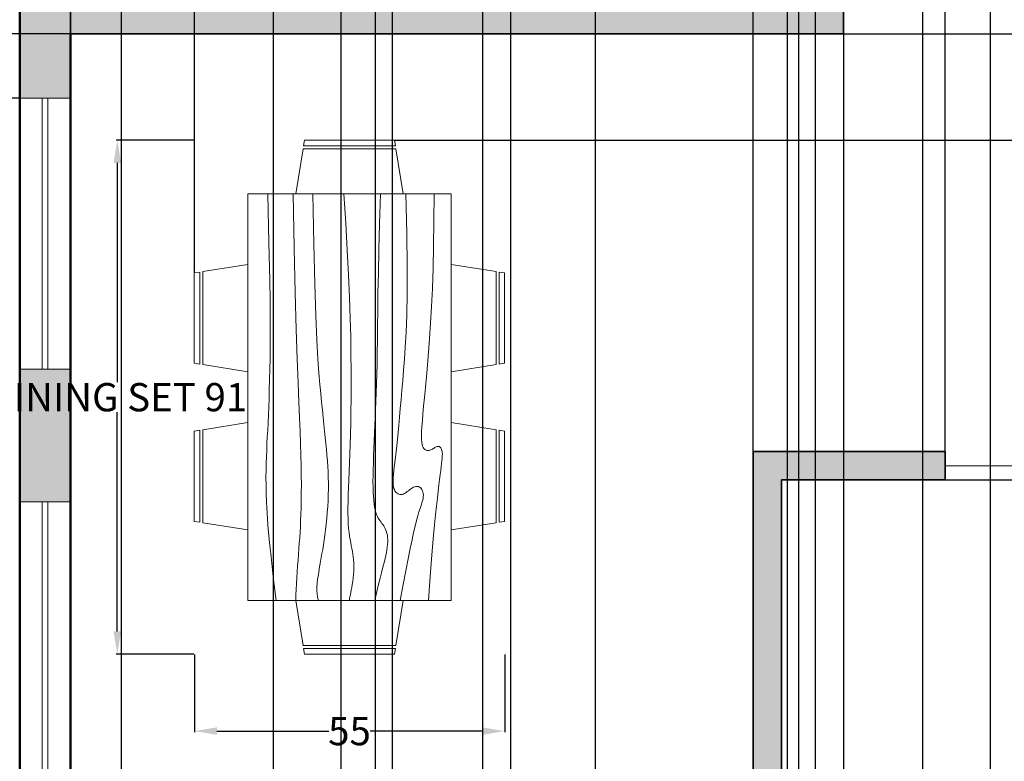
# Model space of a CAD drawing. Units: inches. Extents: x 882 to 1363, y 890 to 1847.
# Tile 4 of 9: x 983 to 1157, y 1220 to 1351. Entities that reach past the tile are written whole.
import ezdxf

# ---------------------------------------------------------------- set-up
doc = ezdxf.new("R2010")
doc.units = ezdxf.units.IN
doc.header["$MEASUREMENT"] = 0
doc.linetypes.add('ACAD_ISO02W100', pattern=[15, 12, -3])
for name, color, linetype, lineweight in [('A-ANNO-DIMS', 2, 'Continuous', 18), ('A-WALL-OVHD', 7, 'ACAD_ISO02W100', 18), ('furniture', 10, 'Continuous', 18), ('inner wall', 50, 'Continuous', 35), ('outer wall', 40, 'Continuous', 50), ('windows', 226, 'Continuous', 18)]:
    doc.layers.add(name, color=color, linetype=linetype, lineweight=lineweight)
doc.layers.add('A-WALL-PATT', color=251, linetype='Continuous', lineweight=13, true_color=0x636466)
doc.styles.get("Standard").update_dxf_attribs({"font": 'arial.ttf'})
doc.dimstyles.get("Standard").update_dxf_attribs({"dimtxt": 5, "dimasz": 4, "dimexe": 0.18, "dimexo": 0.0625, "dimgap": 0.09, "dimtad": 0, "dimtih": 1, "dimtoh": 1, "dimdec": 1, "dimzin": 0, "dimdsep": 46, "dimlunit": 3, "dimtxsty": 'Standard', "dimcen": 0.09, "dimadec": 0, "dimazin": 0, "dimtfac": 1, "dimtdec": 1, "dimtofl": 0, "dimtmove": 0, "dimatfit": 3, "dimfxl": 1, "dimtolj": 1, "dimtzin": 0, "dimarcsym": 0})

# ---------------------------------------------------------------- blocks, each defined once
blk = doc.blocks.new('Dining Set - 36 x 72 in.')
for p, q in [((-22, 27.5), (-22.1562, 26.50042)), ((-5.8416, 26.5), (-22.1534, 26.5)), ((-22, 27.5), (-6, 27.5)), ((-5.8437, 26.49966), (-6, 27.5)), ((6, 27.5), (5.8438, 26.50042)), ((22.1584, 26.5), (5.8466, 26.5)), ((6, 27.5), (22, 27.5)), ((22.1563, 26.49966), (22, 27.5)), ((-22.2343, 26.00059), (-23.4847, 17.99762)), ((-22.2304, 26), (-5.7608, 26)), ((-4.5152, 17.99762), (-5.7655, 25.99926)), ((5.7657, 26.00059), (4.5153, 17.99762)), ((5.7696, 26), (22.2392, 26)), ((23.4848, 17.99762), (22.2345, 25.99926)), ((36, 18), (-36, 18)), ((-36, 18), (-36, -18)), ((36, -18), (36, 18)), ((-44.0006, 8.23428), (-35.9976, 9.48474)), ((44.0006, 8.23428), (35.9976, 9.48474)), ((-45.5, 8), (-44.5004, 8.15617)), ((-45.5, 8), (-45.5, -8)), ((-44.5, -8.15843), (-44.5, 8.15338)), ((-44, 8.23041), (-44, -8.23915)), ((44, 8.23041), (44, -8.23915)), ((44.5, -8.15843), (44.5, 8.15338)), ((45.5, 8), (44.5005, 8.15617)), ((45.5, 8), (45.5, -8)), ((-44.4997, -8.15631), (-45.5, -8)), ((-35.9976, -9.48476), (-43.9993, -8.2345)), ((35.9976, -9.48476), (43.9993, -8.2345)), ((44.4997, -8.15631), (45.5, -8)), ((-36, -18), (36, -18)), ((-22.2343, -26.0006), (-23.4847, -17.99762)), ((-4.5152, -17.99762), (-5.7655, -25.99928)), ((5.7657, -26.0006), (4.5153, -17.99762)), ((23.4848, -17.99762), (22.2345, -25.99928)), ((-22.2304, -26), (-5.7608, -26)), ((5.7696, -26), (22.2392, -26)), ((-22, -27.5), (-22.1562, -26.50044)), ((-5.8416, -26.5), (-22.1534, -26.5)), ((-22, -27.5), (-6, -27.5)), ((-5.8437, -26.49967), (-6, -27.5)), ((6, -27.5), (5.8438, -26.50044)), ((22.1584, -26.5), (5.8466, -26.5)), ((6, -27.5), (22, -27.5)), ((22.1563, -26.49967), (22, -27.5))]:
    blk.add_line(p, q)
for points in [[(-36, 15), (-31.1772, 14.97754), (-26.8079, 14.91406), (-22.8538, 14.81543), (-19.276, 14.6875), (-16.0362, 14.53613), (-13.0957, 14.36718), (-10.4159, 14.18652), (-7.9583, 14), (-5.6904, 13.81315), (-3.6035, 13.63021), (-1.6954, 13.45508), (0.0365, 13.29166), (1.5945, 13.14388), (2.9811, 13.01562), (4.1988, 12.9108), (5.25, 12.83333), (6.1393, 12.78613), (6.8802, 12.76823), (7.4883, 12.77767), (7.9792, 12.8125), (8.3685, 12.87077), (8.6719, 12.95052), (8.9049, 13.0498), (9.0833, 13.16666), (9.2205, 13.29899), (9.3216, 13.44401), (9.3895, 13.59879), (9.4271, 13.76041), (9.4373, 13.92594), (9.4232, 14.09245), (9.3875, 14.257), (9.3333, 14.41666), (9.2638, 14.56917), (9.1836, 14.71484), (9.0975, 14.85465), (9.0104, 14.98958), (8.9272, 15.1206), (8.8529, 15.2487), (8.7922, 15.37483), (8.75, 15.5), (8.7305, 15.62467), (8.7344, 15.74739), (8.7617, 15.86621), (8.8125, 15.97916), (8.8867, 16.08431), (8.9844, 16.17968), (9.1055, 16.26334), (9.25, 16.33333), (9.4189, 16.38802), (9.6172, 16.42708), (9.8506, 16.45052), (10.125, 16.45833), (10.4463, 16.45052), (10.8203, 16.42708), (11.2529, 16.38802), (11.75, 16.33333), (12.3184, 16.26318), (12.9694, 16.17838), (13.7151, 16.07991), (14.5677, 15.96875), (15.5395, 15.84586), (16.6426, 15.71224), (17.8893, 15.56884), (19.2917, 15.41666), (20.859, 15.25667), (22.5879, 15.08984), (24.4721, 14.91715), (26.5052, 14.73958), (28.6809, 14.5581), (30.9929, 14.3737), (33.4347, 14.18733), (36, 14)], [(-36, 10), (-28.9766, 10.14274), (-23.1725, 10.20442), (-18.4241, 10.19775), (-14.5677, 10.13541), (-11.4399, 10.03011), (-8.877, 9.89453), (-6.7154, 9.74137), (-4.7917, 9.58333), (-2.9698, 9.43082), (-1.2246, 9.28515), (0.4415, 9.14534), (2.026, 9.01041), (3.5266, 8.87939), (4.9408, 8.7513), (6.266, 8.62516), (7.5, 8.5), (8.6411, 8.37549), (9.6914, 8.2539), (10.6538, 8.13818), (11.5312, 8.03125), (12.3267, 7.93603), (13.043, 7.85547), (13.6831, 7.79248), (14.25, 7.75), (14.7471, 7.7303), (15.1797, 7.73307), (15.5537, 7.75732), (15.875, 7.80208), (16.1494, 7.86637), (16.3828, 7.94922), (16.5811, 8.04964), (16.75, 8.16666), (16.8944, 8.29915), (17.0143, 8.44531), (17.1089, 8.60319), (17.1771, 8.77083), (17.218, 8.94629), (17.2305, 9.1276), (17.2137, 9.31282), (17.1667, 9.5), (17.0895, 9.6875), (16.987, 9.875), (16.8649, 10.0625), (16.7292, 10.25), (16.5856, 10.4375), (16.4401, 10.625), (16.2985, 10.8125), (16.1667, 11), (16.05, 11.18733), (15.9518, 11.3737), (15.8752, 11.5581), (15.8229, 11.73958), (15.798, 11.91715), (15.8034, 12.08984), (15.842, 12.25667), (15.9167, 12.41666), (16.0295, 12.56836), (16.1784, 12.70833), (16.3605, 12.83268), (16.5729, 12.9375), (16.8127, 13.01888), (17.0768, 13.07291), (17.3625, 13.0957), (17.6667, 13.08333), (17.9894, 13.03312), (18.3418, 12.94726), (18.7382, 12.82918), (19.1927, 12.68229), (19.7195, 12.51001), (20.3327, 12.31575), (21.0465, 12.10294), (21.875, 11.875), (22.8357, 11.63354), (23.959, 11.37304), (25.2786, 11.08618), (26.8282, 10.76562), (28.6414, 10.40405), (30.752, 9.99414), (33.1936, 9.52856), (36, 9)], [(-36, 5.5), (-30.7157, 5.3348), (-26.069, 5.20963), (-21.9946, 5.11767), (-18.4271, 5.05208), (-15.3009, 5.00602), (-12.5508, 4.97265), (-10.1112, 4.94515), (-7.9167, 4.91666), (-5.909, 4.88167), (-4.0586, 4.83984), (-2.3429, 4.79215), (-0.7396, 4.73958), (0.7739, 4.6831), (2.22, 4.6237), (3.6213, 4.56233), (5, 4.5), (6.373, 4.43782), (7.7344, 4.3776), (9.0723, 4.32129), (10.375, 4.27083), (11.6309, 4.22819), (12.8281, 4.19531), (13.9551, 4.17415), (15, 4.16666), (15.954, 4.17448), (16.819, 4.19791), (17.6001, 4.23698), (18.3021, 4.29166), (18.9299, 4.36198), (19.4883, 4.44791), (19.9823, 4.54948), (20.4167, 4.66666), (20.7969, 4.79899), (21.1302, 4.94401), (21.4245, 5.09879), (21.6875, 5.26041), (21.9271, 5.42594), (22.1511, 5.59245), (22.3672, 5.757), (22.5834, 5.91666), (22.8065, 6.06868), (23.0404, 6.21093), (23.2879, 6.34147), (23.5521, 6.45833), (23.8358, 6.55957), (24.142, 6.64323), (24.4735, 6.70735), (24.8334, 6.75), (25.2235, 6.76969), (25.642, 6.76692), (26.0858, 6.74267), (26.5521, 6.69791), (27.0379, 6.63362), (27.5404, 6.55078), (28.0565, 6.45036), (28.5834, 6.33333), (29.1242, 6.19987), (29.7071, 6.04687), (30.3661, 5.87044), (31.1354, 5.66666), (32.0493, 5.43164), (33.142, 5.16146), (34.4475, 4.85221), (36, 4.5)], [(-36, -1), (-30.7915, -0.6591), (-26.0195, -0.38216), (-21.6519, -0.16284), (-17.6563, 0.00521), (-14.0005, 0.12833), (-10.6523, 0.21289), (-7.5796, 0.26522), (-4.75, 0.29166), (-2.134, 0.29793), (0.2878, 0.28711), (2.5317, 0.26163), (4.6146, 0.22396), (6.5529, 0.17651), (8.3633, 0.12174), (10.0623, 0.06209), (11.6667, 0), (13.1899, -0.06201), (14.6341, -0.1211), (15.9982, -0.17432), (17.2813, -0.21875), (18.4823, -0.25147), (19.6003, -0.26953), (20.6343, -0.27002), (21.5834, -0.25), (22.4481, -0.20768), (23.2357, -0.14584), (23.9549, -0.06836), (24.6146, 0.02083), (25.2235, 0.11784), (25.7904, 0.21875), (26.3241, 0.31966), (26.8334, 0.41666), (27.3265, 0.50618), (27.8099, 0.58593), (28.2894, 0.65397), (28.7709, 0.70833), (29.2601, 0.74707), (29.763, 0.76823), (30.2855, 0.76985), (30.8334, 0.75), (31.4088, 0.70784), (31.9994, 0.64713), (32.589, 0.57275), (33.1615, 0.48958), (33.7008, 0.4025), (34.1908, 0.3164), (34.6153, 0.23616), (34.9584, 0.16666), (35.2099, 0.11165), (35.3848, 0.07031), (35.504, 0.04069), (35.5886, 0.02083), (35.6594, 0.00879), (35.7377, 0.0026), (35.8442, 0.00032), (36, 0)], [(-36, -6.5), (-27.1843, -6.31267), (-20.084, -6.1263), (-14.469, -5.9419), (-10.1094, -5.76042), (-6.7752, -5.58285), (-4.2363, -5.41016), (-2.2629, -5.24333), (-0.625, -5.08334), (0.8708, -4.93099), (2.2715, -4.78646), (3.5872, -4.64974), (4.8281, -4.52084), (6.0046, -4.39974), (7.127, -4.28646), (8.2053, -4.18099), (9.25, -4.08334), (10.2705, -3.99382), (11.2734, -3.91407), (12.2647, -3.84603), (13.25, -3.79167), (14.2354, -3.75293), (15.2266, -3.73177), (16.2295, -3.73015), (17.25, -3.75), (18.2912, -3.79248), (19.3451, -3.85547), (20.4009, -3.93604), (21.4479, -4.03125), (22.4754, -4.13819), (23.4727, -4.25391), (24.4289, -4.37549), (25.3334, -4.5), (26.1785, -4.62492), (26.9694, -4.74935), (27.7145, -4.87281), (28.4219, -4.99479), (29.1, -5.11483), (29.7572, -5.23242), (30.4016, -5.34709), (31.0417, -5.45834), (31.6837, -5.56437), (32.3262, -5.65821), (32.9658, -5.73153), (33.599, -5.77604), (34.2224, -5.78345), (34.8327, -5.74545), (35.4264, -5.65373), (36, -5.5)], [(-36, -10), (-26.4022, -9.81299), (-18.4675, -9.62891), (-11.9839, -9.45069), (-6.7396, -9.28125), (-2.5226, -9.12354), (0.8789, -8.98047), (3.6769, -8.85498), (6.0833, -8.75), (8.2767, -8.66765), (10.3021, -8.60677), (12.1712, -8.56543), (13.8958, -8.54167), (15.4876, -8.53353), (16.9583, -8.53907), (18.3197, -8.55632), (19.5834, -8.58334), (20.7616, -8.61841), (21.8685, -8.66081), (22.9188, -8.71004), (23.9271, -8.76563), (24.9081, -8.82707), (25.8763, -8.89388), (26.8465, -8.96558), (27.8334, -9.04167), (28.8474, -9.12118), (29.8828, -9.20117), (30.93, -9.27824), (31.9792, -9.34896), (33.0205, -9.40991), (34.0443, -9.45768), (35.0407, -9.48885), (36, -9.5)], [(-36, -14.5), (-30.0881, -14.33513), (-25.0332, -14.21224), (-20.7312, -14.12647), (-17.0781, -14.07292), (-13.97, -14.04671), (-11.3027, -14.04297), (-8.9724, -14.05681), (-6.875, -14.08334), (-4.9224, -14.11833), (-3.0905, -14.16016), (-1.3709, -14.20785), (0.2448, -14.26042), (1.7647, -14.3169), (3.1973, -14.3763), (4.5507, -14.43767), (5.8333, -14.5), (7.0554, -14.5621), (8.235, -14.62175), (9.3922, -14.67652), (10.5469, -14.72396), (11.7192, -14.76164), (12.929, -14.78711), (14.1965, -14.79794), (15.5417, -14.79167), (16.9933, -14.76424), (18.6152, -14.70508), (20.4804, -14.60197), (22.6615, -14.44271), (25.2312, -14.21509), (28.2624, -13.9069), (31.8277, -13.50594), (36, -13)]]:
    blk.add_lwpolyline(points)
blk = doc.blocks.new('WIN-48IN-9IN')
for p, q in [((4, 0), (4, 48)), ((5, 0), (5, 48))]:
    blk.add_line(p, q)
blk.add_lwpolyline([(0, 48), (9, 48), (9, 0), (0, 0)], close=True)
blk = doc.blocks.new('*D27')
at = {"layer": 'A-ANNO-DIMS', "color": 0, "lineweight": -2, "transparency": 16777216}
for p, q in [((1013.72, 1329.89), (999.96, 1329.89)), ((1000.14, 1325.89), (1000.14, 1287.07)), ((1000.14, 1242.89), (1000.14, 1281.72)), ((1013.72, 1238.89), (999.96, 1238.89))]:
    blk.add_line(p, q, dxfattribs=at)
at = {"layer": 'A-ANNO-DIMS', "color": 0, "transparency": 16777216}
for points in [[(999.47, 1325.89), (1000.8, 1325.89), (1000.14, 1329.89)], [(999.47, 1242.89), (1000.8, 1242.89), (1000.14, 1238.89)]]:
    blk.add_solid(points, dxfattribs=at)
at = {"layer": 'Defpoints', "color": 0, "transparency": 16777216}
for p in [(1013.79, 1329.89), (1000.14, 1238.89), (1013.79, 1238.89)]:
    blk.add_point(p, dxfattribs=at)
at = {"layer": 'A-ANNO-DIMS', "color": 0, "transparency": 16777216, "insert": (1000.14, 1284.39), "char_height": 5, "attachment_point": 5}
blk.add_mtext('\\A1;DINING SET 91', dxfattribs=at)
blk = doc.blocks.new('*D28')
at = {"layer": 'A-ANNO-DIMS', "color": 0, "lineweight": -2, "transparency": 16777216}
for p, q in [((1013.79, 1238.83), (1013.79, 1225.06)), ((1068.79, 1238.83), (1068.79, 1225.06)), ((1017.79, 1225.24), (1037.6, 1225.24)), ((1064.79, 1225.24), (1044.98, 1225.24))]:
    blk.add_line(p, q, dxfattribs=at)
at = {"layer": 'A-ANNO-DIMS', "color": 0, "transparency": 16777216}
for points in [[(1017.79, 1225.91), (1017.79, 1224.58), (1013.79, 1225.24)], [(1064.79, 1225.91), (1064.79, 1224.58), (1068.79, 1225.24)]]:
    blk.add_solid(points, dxfattribs=at)
at = {"layer": 'Defpoints', "color": 0, "transparency": 16777216}
for p in [(1013.79, 1238.89), (1068.79, 1238.89), (1068.79, 1225.24)]:
    blk.add_point(p, dxfattribs=at)
at = {"layer": 'A-ANNO-DIMS', "color": 0, "transparency": 16777216, "insert": (1041.29, 1225.24), "char_height": 5, "attachment_point": 5}
blk.add_mtext('\\A1;55', dxfattribs=at)
blk = doc.blocks.new('*D40')
at = {"layer": 'A-ANNO-DIMS', "color": 0, "lineweight": -2, "transparency": 16777216}
for p, q in [((991.84, 1758.69), (991.84, 893.37)), ((1064.84, 1758.69), (1064.84, 893.37)), ((995.84, 893.55), (1024.69, 893.55)), ((1060.84, 893.55), (1031.99, 893.55))]:
    blk.add_line(p, q, dxfattribs=at)
at = {"layer": 'A-ANNO-DIMS', "color": 0, "transparency": 16777216}
for points in [[(995.84, 894.21), (995.84, 892.88), (991.84, 893.55)], [(1060.84, 894.21), (1060.84, 892.88), (1064.84, 893.55)]]:
    blk.add_solid(points, dxfattribs=at)
at = {"layer": 'Defpoints', "color": 0, "transparency": 16777216}
for p in [(991.84, 1758.75), (1064.84, 1758.75), (1064.84, 893.55)]:
    blk.add_point(p, dxfattribs=at)
at = {"layer": 'A-ANNO-DIMS', "color": 0, "transparency": 16777216, "insert": (1028.34, 893.55), "char_height": 5, "attachment_point": 5}
blk.add_mtext('\\A1;73', dxfattribs=at)
blk = doc.blocks.new('*D41')
at = {"layer": 'A-ANNO-DIMS', "color": 0, "lineweight": -2, "transparency": 16777216}
for p, q in [((1069.84, 1758.69), (1069.84, 893.37)), ((1154.84, 1758.69), (1154.84, 893.37)), ((1073.84, 893.55), (1108.65, 893.55)), ((1150.84, 893.55), (1116.03, 893.55))]:
    blk.add_line(p, q, dxfattribs=at)
at = {"layer": 'A-ANNO-DIMS', "color": 0, "transparency": 16777216}
for points in [[(1073.84, 894.21), (1073.84, 892.88), (1069.84, 893.55)], [(1150.84, 894.21), (1150.84, 892.88), (1154.84, 893.55)]]:
    blk.add_solid(points, dxfattribs=at)
at = {"layer": 'Defpoints', "color": 0, "transparency": 16777216}
for p in [(1069.84, 1758.75), (1154.84, 1758.75), (1154.84, 893.55)]:
    blk.add_point(p, dxfattribs=at)
at = {"layer": 'A-ANNO-DIMS', "color": 0, "transparency": 16777216, "insert": (1112.34, 893.55), "char_height": 5, "attachment_point": 5}
blk.add_mtext('\\A1;85', dxfattribs=at)
blk = doc.blocks.new('*D47')
at = {"layer": 'A-ANNO-DIMS', "color": 0, "lineweight": -2, "transparency": 16777216}
for p, q in [((1123.84, 1567.69), (1123.84, 893.37)), ((1128.84, 1567.69), (1128.84, 893.37)), ((1119.84, 893.55), (1115.84, 893.55)), ((1132.84, 893.55), (1136.84, 893.55))]:
    blk.add_line(p, q, dxfattribs=at)
at = {"layer": 'A-ANNO-DIMS', "color": 0, "transparency": 16777216}
for points in [[(1119.84, 894.21), (1119.84, 892.88), (1123.84, 893.55)], [(1132.84, 894.21), (1132.84, 892.88), (1128.84, 893.55)]]:
    blk.add_solid(points, dxfattribs=at)
at = {"layer": 'Defpoints', "color": 0, "transparency": 16777216}
for p in [(1123.84, 1567.75), (1128.84, 1567.75), (1128.84, 893.55)]:
    blk.add_point(p, dxfattribs=at)
at = {"layer": 'A-ANNO-DIMS', "color": 0, "transparency": 16777216, "insert": (1126.34, 893.55), "char_height": 5, "attachment_point": 5}
blk.add_mtext('\\A1;5', dxfattribs=at)
blk = doc.blocks.new('*D48')
at = {"layer": 'A-ANNO-DIMS', "color": 0, "lineweight": -2, "transparency": 16777216}
for p, q in [((1084.84, 1562.69), (1084.84, 893.37)), ((1120.84, 1562.69), (1120.84, 893.37)), ((1088.84, 893.55), (1099.17, 893.55)), ((1116.84, 893.55), (1106.51, 893.55))]:
    blk.add_line(p, q, dxfattribs=at)
at = {"layer": 'A-ANNO-DIMS', "color": 0, "transparency": 16777216}
for points in [[(1088.84, 894.21), (1088.84, 892.88), (1084.84, 893.55)], [(1116.84, 894.21), (1116.84, 892.88), (1120.84, 893.55)]]:
    blk.add_solid(points, dxfattribs=at)
at = {"layer": 'Defpoints', "color": 0, "transparency": 16777216}
for p in [(1084.84, 1562.75), (1120.84, 1562.75), (1120.84, 893.55)]:
    blk.add_point(p, dxfattribs=at)
at = {"layer": 'A-ANNO-DIMS', "color": 0, "transparency": 16777216, "insert": (1102.84, 893.55), "char_height": 5, "attachment_point": 5}
blk.add_mtext('\\A1;36', dxfattribs=at)
blk = doc.blocks.new('*D51')
at = {"layer": 'A-ANNO-DIMS', "color": 0, "lineweight": -2, "transparency": 16777216}
for p, q in [((982.84, 1767.69), (982.84, 893.37)), ((1000.84, 1767.69), (1000.84, 893.37)), ((986.84, 893.55), (996.84, 893.55)), ((1000.84, 893.55), (1004.84, 893.55))]:
    blk.add_line(p, q, dxfattribs=at)
at = {"layer": 'A-ANNO-DIMS', "color": 0, "transparency": 16777216}
for points in [[(986.84, 894.21), (986.84, 892.88), (982.84, 893.55)], [(996.84, 894.21), (996.84, 892.88), (1000.84, 893.55)]]:
    blk.add_solid(points, dxfattribs=at)
at = {"layer": 'Defpoints', "color": 0, "transparency": 16777216}
for p in [(982.84, 1767.75), (1000.84, 1767.75), (1000.84, 893.55)]:
    blk.add_point(p, dxfattribs=at)
at = {"layer": 'A-ANNO-DIMS', "color": 0, "transparency": 16777216, "insert": (1015.08, 893.55), "char_height": 5, "attachment_point": 5}
blk.add_mtext('\\A1;18.006', dxfattribs=at)
blk = doc.blocks.new('*D52')
at = {"layer": 'A-ANNO-DIMS', "color": 0, "lineweight": -2, "transparency": 16777216}
for p, q in [((1048.84, 1767.69), (1048.84, 893.37)), ((1118.86, 1767.69), (1118.86, 893.37)), ((1052.84, 893.55), (1075.83, 893.55)), ((1114.86, 893.55), (1091.87, 893.55))]:
    blk.add_line(p, q, dxfattribs=at)
at = {"layer": 'A-ANNO-DIMS', "color": 0, "transparency": 16777216}
for points in [[(1052.84, 894.21), (1052.84, 892.88), (1048.84, 893.55)], [(1114.86, 894.21), (1114.86, 892.88), (1118.86, 893.55)]]:
    blk.add_solid(points, dxfattribs=at)
at = {"layer": 'Defpoints', "color": 0, "transparency": 16777216}
for p in [(1048.84, 1767.75), (1118.86, 1767.75), (1118.86, 893.55)]:
    blk.add_point(p, dxfattribs=at)
at = {"layer": 'A-ANNO-DIMS', "color": 0, "transparency": 16777216, "insert": (1083.85, 893.55), "char_height": 5, "attachment_point": 5}
blk.add_mtext('\\A1;70.01', dxfattribs=at)
blk = doc.blocks.new('*D53')
at = {"layer": 'A-ANNO-DIMS', "color": 0, "lineweight": -2, "transparency": 16777216}
for p, q in [((1142.86, 1767.69), (1142.86, 893.37)), ((1171.41, 1767.69), (1171.41, 893.37)), ((1138.86, 893.55), (1134.86, 893.55)), ((1175.41, 893.55), (1179.41, 893.55))]:
    blk.add_line(p, q, dxfattribs=at)
at = {"layer": 'A-ANNO-DIMS', "color": 0, "transparency": 16777216}
for points in [[(1138.86, 894.21), (1138.86, 892.88), (1142.86, 893.55)], [(1175.41, 894.21), (1175.41, 892.88), (1171.41, 893.55)]]:
    blk.add_solid(points, dxfattribs=at)
at = {"layer": 'Defpoints', "color": 0, "transparency": 16777216}
for p in [(1142.86, 1767.75), (1171.41, 1767.75), (1171.41, 893.55)]:
    blk.add_point(p, dxfattribs=at)
at = {"layer": 'A-ANNO-DIMS', "color": 0, "transparency": 16777216, "insert": (1157.14, 893.55), "char_height": 5, "attachment_point": 5}
blk.add_mtext('\\A1;28.554', dxfattribs=at)
blk = doc.blocks.new('*D59')
at = {"layer": 'A-ANNO-DIMS', "color": 0, "lineweight": -2, "transparency": 16777216}
for p, q in [((982.78, 1361.08), (906.46, 1361.08)), ((906.64, 1357.08), (906.64, 1352.75)), ((991.78, 1348.75), (906.46, 1348.75)), ((906.64, 1348.75), (906.64, 1344.75)), ((906.64, 1344.75), (902.64, 1344.75))]:
    blk.add_line(p, q, dxfattribs=at)
at = {"layer": 'A-ANNO-DIMS', "color": 0, "transparency": 16777216}
for points in [[(905.97, 1357.08), (907.3, 1357.08), (906.64, 1361.08)], [(905.97, 1352.75), (907.3, 1352.75), (906.64, 1348.75)]]:
    blk.add_solid(points, dxfattribs=at)
at = {"layer": 'Defpoints', "color": 0, "transparency": 16777216}
for p in [(982.84, 1361.08), (906.64, 1348.75), (991.84, 1348.75)]:
    blk.add_point(p, dxfattribs=at)
at = {"layer": 'A-ANNO-DIMS', "color": 0, "transparency": 16777216, "insert": (892.4, 1344.75), "char_height": 5, "attachment_point": 5}
blk.add_mtext('\\A1;12.328', dxfattribs=at)
blk = doc.blocks.new('*D61')
at = {"layer": 'A-ANNO-DIMS', "color": 0, "lineweight": -2, "transparency": 16777216}
for p, q in [((991.84, 1348.69), (991.84, 893.37)), ((1128.84, 1348.69), (1128.84, 893.37)), ((995.84, 893.55), (1054.96, 893.55)), ((1124.84, 893.55), (1065.72, 893.55))]:
    blk.add_line(p, q, dxfattribs=at)
at = {"layer": 'A-ANNO-DIMS', "color": 0, "transparency": 16777216}
for points in [[(995.84, 894.21), (995.84, 892.88), (991.84, 893.55)], [(1124.84, 894.21), (1124.84, 892.88), (1128.84, 893.55)]]:
    blk.add_solid(points, dxfattribs=at)
at = {"layer": 'Defpoints', "color": 0, "transparency": 16777216}
for p in [(991.84, 1348.75), (1128.84, 1348.75), (1128.84, 893.55)]:
    blk.add_point(p, dxfattribs=at)
at = {"layer": 'A-ANNO-DIMS', "color": 0, "transparency": 16777216, "insert": (1060.34, 893.55), "char_height": 5, "attachment_point": 5}
blk.add_mtext('\\A1;137', dxfattribs=at)
blk = doc.blocks.new('*D62')
at = {"layer": 'A-ANNO-DIMS', "color": 0, "lineweight": -2, "transparency": 16777216}
for p, q in [((991.9, 1348.75), (1353.22, 1348.75)), ((1353.04, 1344.75), (1353.04, 1230.35)), ((1353.04, 1110.75), (1353.04, 1225.15)), ((991.9, 1106.75), (1353.22, 1106.75))]:
    blk.add_line(p, q, dxfattribs=at)
at = {"layer": 'A-ANNO-DIMS', "color": 0, "transparency": 16777216}
for points in [[(1352.38, 1344.75), (1353.71, 1344.75), (1353.04, 1348.75)], [(1352.38, 1110.75), (1353.71, 1110.75), (1353.04, 1106.75)]]:
    blk.add_solid(points, dxfattribs=at)
at = {"layer": 'Defpoints', "color": 0, "transparency": 16777216}
for p in [(991.84, 1348.75), (991.84, 1106.75), (1353.04, 1106.75)]:
    blk.add_point(p, dxfattribs=at)
at = {"layer": 'A-ANNO-DIMS', "color": 0, "transparency": 16777216, "insert": (1353.04, 1227.75), "char_height": 5, "attachment_point": 5}
blk.add_mtext('\\A1;242', dxfattribs=at)
blk = doc.blocks.new('*D64')
at = {"layer": 'A-ANNO-DIMS', "color": 0, "lineweight": -2, "transparency": 16777216}
for p, q in [((1117.84, 1269.69), (1117.84, 893.37)), ((1243.84, 1269.69), (1243.84, 893.37)), ((1121.84, 893.55), (1175.46, 893.55)), ((1239.84, 893.55), (1186.22, 893.55))]:
    blk.add_line(p, q, dxfattribs=at)
at = {"layer": 'A-ANNO-DIMS', "color": 0, "transparency": 16777216}
for points in [[(1121.84, 894.21), (1121.84, 892.88), (1117.84, 893.55)], [(1239.84, 894.21), (1239.84, 892.88), (1243.84, 893.55)]]:
    blk.add_solid(points, dxfattribs=at)
at = {"layer": 'Defpoints', "color": 0, "transparency": 16777216}
for p in [(1117.84, 1269.75), (1243.84, 1269.75), (1243.84, 893.55)]:
    blk.add_point(p, dxfattribs=at)
at = {"layer": 'A-ANNO-DIMS', "color": 0, "transparency": 16777216, "insert": (1180.84, 893.55), "char_height": 5, "attachment_point": 5}
blk.add_mtext('\\A1;126', dxfattribs=at)
blk = doc.blocks.new('*D65')
at = {"layer": 'A-ANNO-DIMS', "color": 0, "lineweight": -2, "transparency": 16777216}
for p, q in [((1117.9, 1269.75), (1353.22, 1269.75)), ((1353.04, 1265.75), (1353.04, 1212.39)), ((1353.04, 1153.75), (1353.04, 1207.11)), ((1117.9, 1149.75), (1353.22, 1149.75))]:
    blk.add_line(p, q, dxfattribs=at)
at = {"layer": 'A-ANNO-DIMS', "color": 0, "transparency": 16777216}
for points in [[(1352.38, 1265.75), (1353.71, 1265.75), (1353.04, 1269.75)], [(1352.38, 1153.75), (1353.71, 1153.75), (1353.04, 1149.75)]]:
    blk.add_solid(points, dxfattribs=at)
at = {"layer": 'Defpoints', "color": 0, "transparency": 16777216}
for p in [(1117.84, 1269.75), (1353.04, 1269.75), (1117.84, 1149.75)]:
    blk.add_point(p, dxfattribs=at)
at = {"layer": 'A-ANNO-DIMS', "color": 0, "transparency": 16777216, "insert": (1353.04, 1209.75), "char_height": 5, "attachment_point": 5}
blk.add_mtext('\\A1;120', dxfattribs=at)
blk = doc.blocks.new('*D68')
at = {"layer": 'A-ANNO-DIMS', "color": 0, "lineweight": -2, "transparency": 16777216}
for p, q in [((1027.84, 1142.81), (1027.84, 1844.13)), ((1031.84, 1843.95), (1066.65, 1843.95)), ((1108.84, 1843.95), (1074.03, 1843.95)), ((1112.84, 1142.81), (1112.84, 1844.13))]:
    blk.add_line(p, q, dxfattribs=at)
at = {"layer": 'A-ANNO-DIMS', "color": 0, "transparency": 16777216}
for points in [[(1031.84, 1844.62), (1031.84, 1843.29), (1027.84, 1843.95)], [(1108.84, 1844.62), (1108.84, 1843.29), (1112.84, 1843.95)]]:
    blk.add_solid(points, dxfattribs=at)
at = {"layer": 'Defpoints', "color": 0, "transparency": 16777216}
for p in [(1112.84, 1843.95), (1027.84, 1142.75), (1112.84, 1142.75)]:
    blk.add_point(p, dxfattribs=at)
at = {"layer": 'A-ANNO-DIMS', "color": 0, "transparency": 16777216, "insert": (1070.34, 1843.95), "char_height": 5, "attachment_point": 5}
blk.add_mtext('\\A1;85', dxfattribs=at)
blk = doc.blocks.new('*D74')
at = {"layer": 'A-ANNO-DIMS', "color": 0, "lineweight": -2, "transparency": 16777216}
for p, q in [((991.84, 1002.81), (991.84, 1844.13)), ((995.84, 1843.95), (1012.06, 1843.95)), ((1035.84, 1843.95), (1019.62, 1843.95)), ((1039.84, 1002.81), (1039.84, 1844.13))]:
    blk.add_line(p, q, dxfattribs=at)
at = {"layer": 'A-ANNO-DIMS', "color": 0, "transparency": 16777216}
for points in [[(995.84, 1844.62), (995.84, 1843.29), (991.84, 1843.95)], [(1035.84, 1844.62), (1035.84, 1843.29), (1039.84, 1843.95)]]:
    blk.add_solid(points, dxfattribs=at)
at = {"layer": 'Defpoints', "color": 0, "transparency": 16777216}
for p in [(1039.84, 1843.95), (991.84, 1002.75), (1039.84, 1002.75)]:
    blk.add_point(p, dxfattribs=at)
at = {"layer": 'A-ANNO-DIMS', "color": 0, "transparency": 16777216, "insert": (1015.84, 1843.95), "char_height": 5, "attachment_point": 5}
blk.add_mtext('\\A1;48', dxfattribs=at)
blk = doc.blocks.new('*D78')
at = {"layer": 'A-ANNO-DIMS', "color": 0, "lineweight": -2, "transparency": 16777216}
for p, q in [((1146.84, 1274.81), (1146.84, 1844.13)), ((1150.84, 1843.95), (1179.69, 1843.95)), ((1215.84, 1843.95), (1186.99, 1843.95)), ((1219.84, 1274.81), (1219.84, 1844.13))]:
    blk.add_line(p, q, dxfattribs=at)
at = {"layer": 'A-ANNO-DIMS', "color": 0, "transparency": 16777216}
for points in [[(1150.84, 1844.62), (1150.84, 1843.29), (1146.84, 1843.95)], [(1215.84, 1844.62), (1215.84, 1843.29), (1219.84, 1843.95)]]:
    blk.add_solid(points, dxfattribs=at)
at = {"layer": 'Defpoints', "color": 0, "transparency": 16777216}
for p in [(1219.84, 1843.95), (1146.84, 1274.75), (1219.84, 1274.75)]:
    blk.add_point(p, dxfattribs=at)
at = {"layer": 'A-ANNO-DIMS', "color": 0, "transparency": 16777216, "insert": (1183.34, 1843.95), "char_height": 5, "attachment_point": 5}
blk.add_mtext('\\A1;73', dxfattribs=at)
blk = doc.blocks.new('*D83')
at = {"layer": 'A-ANNO-DIMS', "color": 0, "lineweight": -2, "transparency": 16777216}
for p, q in [((906.64, 1348.75), (906.64, 1352.75)), ((906.64, 1352.75), (910.64, 1352.75)), ((991.78, 1348.75), (906.46, 1348.75)), ((906.64, 1341.33), (906.64, 1344.75)), ((982.78, 1337.33), (906.46, 1337.33))]:
    blk.add_line(p, q, dxfattribs=at)
at = {"layer": 'A-ANNO-DIMS', "color": 0, "transparency": 16777216}
for points in [[(905.97, 1344.75), (907.3, 1344.75), (906.64, 1348.75)], [(905.97, 1341.33), (907.3, 1341.33), (906.64, 1337.33)]]:
    blk.add_solid(points, dxfattribs=at)
at = {"layer": 'Defpoints', "color": 0, "transparency": 16777216}
for p in [(906.64, 1348.75), (991.84, 1348.75), (982.84, 1337.33)]:
    blk.add_point(p, dxfattribs=at)
at = {"layer": 'A-ANNO-DIMS', "color": 0, "transparency": 16777216, "insert": (920.87, 1352.75), "char_height": 5, "attachment_point": 5}
blk.add_mtext('\\A1;11.416', dxfattribs=at)
blk = doc.blocks.new('*D85')
at = {"layer": 'A-ANNO-DIMS', "color": 0, "lineweight": -2, "transparency": 16777216}
for p, q in [((1045.84, 1562.69), (1045.84, 893.37)), ((1084.84, 1562.69), (1084.84, 893.37)), ((1049.84, 893.55), (1061.66, 893.55)), ((1080.84, 893.55), (1069.01, 893.55))]:
    blk.add_line(p, q, dxfattribs=at)
at = {"layer": 'A-ANNO-DIMS', "color": 0, "transparency": 16777216}
for points in [[(1049.84, 894.21), (1049.84, 892.88), (1045.84, 893.55)], [(1080.84, 894.21), (1080.84, 892.88), (1084.84, 893.55)]]:
    blk.add_solid(points, dxfattribs=at)
at = {"layer": 'Defpoints', "color": 0, "transparency": 16777216}
for p in [(1045.84, 1562.75), (1084.84, 1562.75), (1084.84, 893.55)]:
    blk.add_point(p, dxfattribs=at)
at = {"layer": 'A-ANNO-DIMS', "color": 0, "transparency": 16777216, "insert": (1065.34, 893.55), "char_height": 5, "attachment_point": 5}
blk.add_mtext('\\A1;39', dxfattribs=at)
blk = doc.blocks.new('*D88')
at = {"layer": 'A-ANNO-DIMS', "color": 0, "lineweight": -2, "transparency": 16777216}
for p, q in [((1128.84, 1567.69), (1128.84, 893.37)), ((1211.84, 1562.69), (1211.84, 893.37)), ((1132.84, 893.55), (1166.66, 893.55)), ((1207.84, 893.55), (1174.01, 893.55))]:
    blk.add_line(p, q, dxfattribs=at)
at = {"layer": 'A-ANNO-DIMS', "color": 0, "transparency": 16777216}
for points in [[(1132.84, 894.21), (1132.84, 892.88), (1128.84, 893.55)], [(1207.84, 894.21), (1207.84, 892.88), (1211.84, 893.55)]]:
    blk.add_solid(points, dxfattribs=at)
at = {"layer": 'Defpoints', "color": 0, "transparency": 16777216}
for p in [(1128.84, 1567.75), (1211.84, 1562.75), (1211.84, 893.55)]:
    blk.add_point(p, dxfattribs=at)
at = {"layer": 'A-ANNO-DIMS', "color": 0, "transparency": 16777216, "insert": (1170.34, 893.55), "char_height": 5, "attachment_point": 5}
blk.add_mtext('\\A1;83', dxfattribs=at)
blk = doc.blocks.new('*D89')
at = {"layer": 'A-ANNO-DIMS', "color": 0, "lineweight": -2, "transparency": 16777216}
for p, q in [((991.84, 1473.69), (991.84, 893.37)), ((1084.84, 1473.69), (1084.84, 893.37)), ((995.84, 893.55), (1034.67, 893.55)), ((1080.84, 893.55), (1042.01, 893.55))]:
    blk.add_line(p, q, dxfattribs=at)
at = {"layer": 'A-ANNO-DIMS', "color": 0, "transparency": 16777216}
for points in [[(995.84, 894.21), (995.84, 892.88), (991.84, 893.55)], [(1080.84, 894.21), (1080.84, 892.88), (1084.84, 893.55)]]:
    blk.add_solid(points, dxfattribs=at)
at = {"layer": 'Defpoints', "color": 0, "transparency": 16777216}
for p in [(991.84, 1473.75), (1084.84, 1473.75), (1084.84, 893.55)]:
    blk.add_point(p, dxfattribs=at)
at = {"layer": 'A-ANNO-DIMS', "color": 0, "transparency": 16777216, "insert": (1038.34, 893.55), "char_height": 5, "attachment_point": 5}
blk.add_mtext('\\A1;93', dxfattribs=at)
blk = doc.blocks.new('*D93')
at = {"layer": 'A-ANNO-DIMS', "color": 0, "lineweight": -2, "transparency": 16777216}
for p, q in [((987.84, 1843.95), (983.84, 1843.95)), ((991.84, 1337.4), (991.84, 1844.13)), ((1013.79, 1306.45), (1013.79, 1844.13)), ((1017.79, 1843.95), (1021.79, 1843.95))]:
    blk.add_line(p, q, dxfattribs=at)
at = {"layer": 'A-ANNO-DIMS', "color": 0, "transparency": 16777216}
for points in [[(987.84, 1844.62), (987.84, 1843.29), (991.84, 1843.95)], [(1017.79, 1844.62), (1017.79, 1843.29), (1013.79, 1843.95)]]:
    blk.add_solid(points, dxfattribs=at)
at = {"layer": 'Defpoints', "color": 0, "transparency": 16777216}
for p in [(1013.79, 1843.95), (991.84, 1337.33), (1013.79, 1306.39)]:
    blk.add_point(p, dxfattribs=at)
at = {"layer": 'A-ANNO-DIMS', "color": 0, "transparency": 16777216, "insert": (1002.81, 1843.95), "char_height": 5, "attachment_point": 5}
blk.add_mtext('\\A1;21.95', dxfattribs=at)
blk = doc.blocks.new('*D94')
at = {"layer": 'A-ANNO-DIMS', "color": 0, "lineweight": -2, "transparency": 16777216}
for p, q in [((1128.9, 1348.75), (1353.22, 1348.75)), ((1353.04, 1344.75), (1353.04, 1341.96)), ((1353.04, 1333.89), (1353.04, 1336.68)), ((1049.35, 1329.89), (1353.22, 1329.89))]:
    blk.add_line(p, q, dxfattribs=at)
at = {"layer": 'A-ANNO-DIMS', "color": 0, "transparency": 16777216}
for points in [[(1352.38, 1344.75), (1353.71, 1344.75), (1353.04, 1348.75)], [(1352.38, 1333.89), (1353.71, 1333.89), (1353.04, 1329.89)]]:
    blk.add_solid(points, dxfattribs=at)
at = {"layer": 'Defpoints', "color": 0, "transparency": 16777216}
for p in [(1128.84, 1348.75), (1353.04, 1348.75), (1049.29, 1329.89)]:
    blk.add_point(p, dxfattribs=at)
at = {"layer": 'A-ANNO-DIMS', "color": 0, "transparency": 16777216, "insert": (1353.04, 1339.32), "char_height": 5, "attachment_point": 5}
blk.add_mtext('\\A1;18.858', dxfattribs=at)

msp = doc.modelspace()

# ---------------------------------------------------------------- hatches: boundary and pattern name
at = {"layer": 'A-WALL-PATT'}
h = msp.add_hatch(color=256, dxfattribs=at)
h.dxf.hatch_style = 1
h.paths.add_polyline_path([(1050.8388, 1481.7495), (1050.8388, 1478.7495), (1084.8388, 1478.7495), (1084.8388, 1473.7495), (991.8388, 1473.7495), (991.8388, 1361.0778), (982.8388, 1361.0778), (982.8388, 1556.1531), (991.8388, 1556.1531), (991.8388, 1478.7495), (1045.8388, 1478.7495), (1045.8388, 1481.7479), (1045.4161, 1481.7477), (1030.9055, 1506.8563), (1032.004, 1507.4911), (1046.5146, 1482.3825), (1045.4161, 1481.7477), (1045.8388, 1481.7479), (1045.8388, 1481.7495)])
h.paths.add_polyline_path([(1128.8388, 1478.7495), (1120.8388, 1478.7495), (1120.8388, 1473.7495), (1123.8388, 1473.7495), (1123.8388, 1353.7495), (991.8388, 1353.7495), (991.8388, 1361.0778), (982.8388, 1361.0778), (982.8388, 1337.3333), (991.8388, 1337.3333), (991.8388, 1348.7495), (1128.8388, 1348.7495)])
h.paths.add_polyline_path([(1118.8585, 1767.7495), (1048.8447, 1767.7495), (1048.8447, 1758.7495), (1064.8388, 1758.7495), (1069.8388, 1758.7495), (1118.8585, 1758.7495)])
h.paths.add_polyline_path([(1171.4129, 1767.7495), (1142.8585, 1767.7495), (1142.8585, 1758.7495), (1154.8388, 1758.7495), (1154.8388, 1710.7495), (1069.8388, 1710.7495), (1069.8388, 1713.7495), (1064.8388, 1713.7495), (1064.8388, 1705.7495), (1123.8388, 1705.7495), (1123.8388, 1567.7495), (1120.8388, 1567.7495), (1120.8388, 1562.7495), (1123.8388, 1562.7495), (1211.8388, 1562.7495), (1211.8388, 1567.7495), (1128.8388, 1567.7495), (1128.8388, 1705.7495), (1211.8388, 1705.7495), (1211.8388, 1710.7495), (1159.8388, 1710.7495), (1159.8388, 1758.7495), (1171.4129, 1758.7495)])
h.paths.add_polyline_path([(1252.8388, 1767.7495), (1195.4129, 1767.7495), (1195.4129, 1758.7495), (1243.8388, 1758.7495), (1243.8388, 1710.7495), (1240.8388, 1710.7495), (1240.8388, 1706.4648), (1240.8388, 1705.7495), (1243.8388, 1705.7495), (1243.8388, 1673.1735), (1252.8388, 1673.1735)])
h.paths.add_polyline_path([(1252.8388, 1625.1735), (1243.8388, 1625.1735), (1243.8388, 1567.7495), (1240.8388, 1567.7495), (1240.8388, 1562.7495), (1243.8388, 1562.7495), (1243.8388, 1546.029), (1252.8388, 1546.029)])
h.paths.add_polyline_path([(1252.8388, 1498.029), (1243.8388, 1498.029), (1243.8388, 1391.1399), (1252.8388, 1391.1399)])
h.paths.add_polyline_path([(1252.8388, 1179.8561), (1243.8388, 1179.8561), (1243.8388, 1149.7495), (1219.8388, 1149.7495), (1219.8388, 1145.3111), (1219.8388, 1144.7495), (1252.8388, 1144.7495)])
h.paths.add_polyline_path([(1252.8388, 1277.7495), (1243.8388, 1277.7495), (1243.8388, 1274.7495), (1219.8388, 1274.7495), (1219.8388, 1269.7495), (1243.8388, 1269.7495), (1243.8388, 1227.8561), (1252.8388, 1227.8561)])
h.paths.add_polyline_path([(1252.8388, 1343.1399), (1243.8388, 1343.1399), (1243.8388, 1313.7495), (1248.3388, 1313.7495), (1252.8388, 1313.7495)])
h.paths.add_polyline_path([(1146.8388, 1274.7495), (1112.8388, 1274.7495), (1112.8388, 1106.7495), (1106.7761, 1106.7495), (1106.7761, 1101.7495), (1117.8388, 1101.7495), (1117.8388, 1144.7495), (1159.8388, 1144.7495), (1159.8388, 1149.7495), (1117.8388, 1149.7495), (1117.8388, 1269.7495), (1146.8388, 1269.7495)])
h = msp.add_hatch(color=256, dxfattribs=at)
h.dxf.hatch_style = 1
h.paths.add_polyline_path([(1000.8447, 1767.7495), (993.3979, 1767.7495), (991.8388, 1758.7495), (1000.8447, 1758.7495)])
h.paths.add_polyline_path([(991.8388, 1654.8981), (982.8388, 1654.3544), (982.8388, 1595.0521), (991.8388, 1594.8981)])
h.paths.add_polyline_path([(991.8388, 1594.8981), (982.8388, 1595.0521), (982.8388, 1559.7196), (991.8388, 1562.7495), (991.8388, 1567.7495)])
h.paths.add_polyline_path([(991.8388, 1562.7495), (982.8388, 1559.7196), (982.8388, 1556.1531), (991.8388, 1556.1531)])
h.paths.add_polyline_path([(991.8388, 1289.3333), (982.8388, 1289.3333), (982.8388, 1265.8272), (991.8388, 1265.8272)])
h.paths.add_polyline_path([(1058.7761, 1106.7495), (991.8388, 1106.7495), (982.8388, 1107.8066), (982.8388, 1101.3439), (991.8388, 1101.7495), (1058.7761, 1101.7495)])

# ---------------------------------------------------------------- linework, layer by layer
at = {"layer": 'A-WALL-OVHD'}
msp.add_line((1146.8388, 1272.2495), (1219.8388, 1272.2495), dxfattribs=at)
at = {"layer": 'inner wall'}
for p, q in [((1128.8388, 1348.7495), (1128.8388, 1478.7495)), ((991.8388, 1348.7495), (1128.8388, 1348.7495)), ((1112.8388, 1274.7495), (1146.8388, 1274.7495)), ((1112.8388, 1274.7495), (1112.8388, 1106.7495)), ((1146.8388, 1274.7495), (1146.8388, 1269.7495)), ((1117.8388, 1269.7495), (1146.8388, 1269.7495)), ((1117.8388, 1269.7495), (1117.8388, 1149.7495))]:
    msp.add_line(p, q, dxfattribs=at)
at = {"layer": 'outer wall'}
for p, q in [((982.8388, 993.7495), (982.8388, 1767.7495)), ((991.8388, 1106.7495), (991.8388, 1348.7495))]:
    msp.add_line(p, q, dxfattribs=at)

# ---------------------------------------------------------------- block references
at = {"layer": 'furniture', "rotation": 270}
msp.add_blockref('Dining Set - 36 x 72 in.', (1041.2874, 1284.3919), dxfattribs=at)
at = {"layer": 'windows'}
for p in [(982.839, 1289.3335), (982.839, 1217.8274)]:
    msp.add_blockref('WIN-48IN-9IN', p, dxfattribs=at)

# ---------------------------------------------------------------- dimensions: what is measured, and where the dimension line sits
at = {"layer": 'A-ANNO-DIMS'}
for base, p1, p2, override, picture, middle in [((1013.7874, 1843.953), (991.8388, 1337.3333), (1013.7874, 1306.3919), {"dimdec": 2, "dimlfac": 1, "dimrnd": 0, "dimzin": 0, "dimdsep": 46, "dimlunit": 2}, '*D93', (1002.8131, 1843.953)), ((1039.8388, 1843.953), (991.8388, 1002.7495), (1039.8388, 1002.7495), {"dimdec": 0, "dimlfac": 1, "dimrnd": 0, "dimzin": 0, "dimdsep": 46, "dimlunit": 2}, '*D74', (1015.8388, 1843.953)), ((1112.8388, 1843.953), (1027.8388, 1142.7495), (1112.8388, 1142.7495), {"dimdec": 0, "dimlfac": 1, "dimrnd": 0, "dimzin": 0, "dimdsep": 46, "dimlunit": 2}, '*D68', (1070.3388, 1843.953)), ((1219.8388, 1843.953), (1146.8388, 1274.7495), (1219.8388, 1274.7495), {"dimdec": 0, "dimlfac": 1, "dimrnd": 0, "dimzin": 0, "dimdsep": 46, "dimlunit": 2}, '*D78', (1183.3388, 1843.953)), ((1000.8447, 893.546), (982.8388, 1767.7495), (1000.8447, 1767.7495), {"dimdec": 3, "dimlfac": 1, "dimrnd": 0, "dimzin": 0, "dimdsep": 46, "dimlunit": 2}, '*D51', (1015.0762, 893.546)), ((1118.8585, 893.546), (1048.8447, 1767.7495), (1118.8585, 1767.7495), {"dimdec": 2, "dimlfac": 1, "dimrnd": 0, "dimzin": 0, "dimdsep": 46, "dimlunit": 2}, '*D52', (1083.8516, 893.546)), ((1171.4129, 893.546), (1142.8585, 1767.7495), (1171.4129, 1767.7495), {"dimdec": 3, "dimlfac": 1, "dimrnd": 0, "dimzin": 0, "dimdsep": 46, "dimlunit": 2}, '*D53', (1157.1357, 893.546)), ((1064.8388, 893.546), (991.8388, 1758.7495), (1064.8388, 1758.7495), {"dimdec": 0, "dimlfac": 1, "dimrnd": 0, "dimzin": 0, "dimdsep": 46, "dimlunit": 2}, '*D40', (1028.3388, 893.546)), ((1154.8388, 893.546), (1069.8388, 1758.7495), (1154.8388, 1758.7495), {"dimdec": 0, "dimlfac": 1, "dimrnd": 0, "dimzin": 0, "dimdsep": 46, "dimlunit": 2}, '*D41', (1112.3388, 893.546)), ((1128.8388, 893.546), (1123.8388, 1567.7495), (1128.8388, 1567.7495), {"dimdec": 0, "dimlfac": 1, "dimrnd": 0, "dimzin": 0, "dimdsep": 46, "dimlunit": 2}, '*D47', (1126.3388, 893.546)), ((1211.8388, 893.546), (1128.8388, 1567.7495), (1211.8388, 1562.7495), {"dimdec": 0, "dimlfac": 1, "dimrnd": 0, "dimzin": 0, "dimdsep": 46, "dimlunit": 2}, '*D88', (1170.3388, 893.546)), ((1084.8388, 893.546), (1045.8388, 1562.7495), (1084.8388, 1562.7495), {"dimdec": 0, "dimlfac": 1, "dimrnd": 0, "dimzin": 0, "dimdsep": 46, "dimlunit": 2}, '*D85', (1065.3388, 893.546)), ((1120.8388, 893.546), (1084.8388, 1562.7495), (1120.8388, 1562.7495), {"dimdec": 0, "dimlfac": 1, "dimrnd": 0, "dimzin": 0, "dimdsep": 46, "dimlunit": 2}, '*D48', (1102.8388, 893.546)), ((1084.8388, 893.546), (991.8388, 1473.7495), (1084.8388, 1473.7495), {"dimdec": 0, "dimlfac": 1, "dimrnd": 0, "dimzin": 0, "dimdsep": 46, "dimlunit": 2}, '*D89', (1038.3388, 893.546)), ((1128.8388, 893.546), (991.8388, 1348.7495), (1128.8388, 1348.7495), {"dimdec": 0, "dimlfac": 1, "dimrnd": 0, "dimzin": 0, "dimdsep": 46, "dimlunit": 2}, '*D61', (1060.3388, 893.546)), ((1243.8388, 893.546), (1117.8388, 1269.7495), (1243.8388, 1269.7495), {"dimdec": 0, "dimlfac": 1, "dimrnd": 0, "dimzin": 0, "dimdsep": 46, "dimlunit": 2}, '*D64', (1180.8388, 893.546)), ((1068.7874, 1225.2419), (1013.7874, 1238.8919), (1068.7874, 1238.8919), {"dimdec": 0, "dimlfac": 1, "dimrnd": 0, "dimzin": 0, "dimdsep": 46, "dimlunit": 2}, '*D28', (1041.2874, 1225.2419))]:
    dim = msp.add_linear_dim(base=base, p1=p1, p2=p2, dimstyle='Standard', override=override, dxfattribs=at)
    dim.commit()
    dim.dimension.update_dxf_attribs({"geometry": picture, "text_midpoint": middle})
for base, p1, p2, override, picture, middle in [((906.6353, 1348.7495), (982.8388, 1361.0778), (991.8388, 1348.7495), {"dimdec": 3, "dimlfac": 1, "dimrnd": 0, "dimzin": 0, "dimdsep": 46, "dimlunit": 2}, '*D59', (892.397, 1344.7495)), ((906.6353, 1348.7495), (982.8388, 1337.3333), (991.8388, 1348.7495), {"dimdec": 3, "dimlfac": 1, "dimrnd": 0, "dimzin": 0, "dimdsep": 46, "dimlunit": 2}, '*D83', (920.8669, 1352.7495)), ((1353.0423, 1106.7495), (991.8388, 1348.7495), (991.8388, 1106.7495), {"dimdec": 0, "dimlfac": 1, "dimrnd": 0, "dimzin": 0, "dimdsep": 46, "dimlunit": 2}, '*D62', (1353.0423, 1227.7495)), ((1353.0423, 1348.7495), (1049.2874, 1329.8919), (1128.8388, 1348.7495), {"dimdec": 3, "dimlfac": 1, "dimrnd": 0, "dimzin": 0, "dimdsep": 46, "dimlunit": 2}, '*D94', (1353.0423, 1339.3207)), ((1353.0423, 1269.7495), (1117.8388, 1149.7495), (1117.8388, 1269.7495), {"dimdec": 0, "dimlfac": 1, "dimrnd": 0, "dimzin": 0, "dimdsep": 46, "dimlunit": 2}, '*D65', (1353.0423, 1209.7495))]:
    dim = msp.add_linear_dim(base=base, p1=p1, p2=p2, angle=90, dimstyle='Standard', override=override, dxfattribs=at)
    dim.commit()
    dim.dimension.update_dxf_attribs({"geometry": picture, "text_midpoint": middle})
dim = msp.add_linear_dim(base=(1000.1374, 1238.8919), p1=(1013.7874, 1329.8919), p2=(1013.7874, 1238.8919), angle=270, text='DINING SET <>', dimstyle='Standard', override={"dimdec": 0, "dimlfac": 1, "dimrnd": 0, "dimzin": 0, "dimdsep": 46, "dimlunit": 2}, dxfattribs=at)
dim.commit()
dim.dimension.update_dxf_attribs({"geometry": '*D27', "text_midpoint": (1000.1374, 1284.3919)})

doc.saveas('drawing.dxf')
